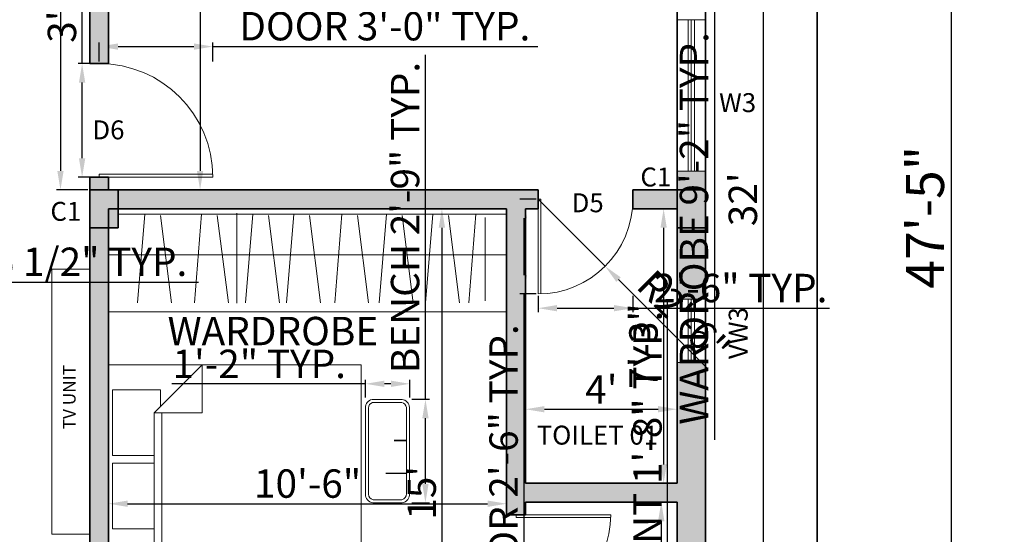
# Model space of a CAD drawing. Units: inches. Extents: x 4312 to 4955, y 6030 to 6717.
# Tile 3 of 5: x 4643 to 4955, y 6255 to 6418. Entities that reach past the tile are written whole.
import ezdxf

# ---------------------------------------------------------------- set-up
doc = ezdxf.new("R2010")
doc.units = ezdxf.units.IN
for name, color, linetype, lineweight in [('A-AREA-IDEN', 7, 'Continuous', 20), ('A-FLOR-CASE', 40, 'Continuous', 18), ('A-WALL', 7, 'Continuous', 35), ('C-PROP', 7, 'Continuous', 35), ('Dimensions', 112, 'Continuous', 13), ('Doors', 10, 'Continuous', 18), ('Furniture', 30, 'Continuous', 18), ('Text', 30, 'Continuous', 18), ('Windows', 160, 'Continuous', 18)]:
    doc.layers.add(name, color=color, linetype=linetype, lineweight=lineweight)
doc.layers.add('A-WALL-PATT', color=251, linetype='Continuous', lineweight=13, true_color=0x636466)
doc.layers.add('Column', color=52, linetype='Continuous', lineweight=35, true_color=0xc8c92d)
doc.styles.get("Standard").update_dxf_attribs({"font": 'arial.ttf'})
doc.dimstyles.new('ISO-25', dxfattribs={"dimtxt": 9, "dimasz": 6, "dimexe": 1.25, "dimexo": 0.625, "dimtad": 1, "dimdec": 1, "dimlunit": 3, "dimtxsty": 'Standard', "dimcen": 2.5, "dimadec": 0, "dimazin": 0, "dimtfac": 1, "dimtdec": 1, "dimtmove": 0, "dimatfit": 3, "dimfxl": 1, "dimarcsym": 0})

# ---------------------------------------------------------------- blocks, each defined once
blk = doc.blocks.new('D2')
at = {"layer": 'Doors'}
for p, q in [((4718.9, 6093.56), (4754.9, 6093.56)), ((4718.9, 6092.56), (4718.9, 6093.56)), ((4718.9, 6092.56), (4754.9, 6092.56))]:
    blk.add_line(p, q, dxfattribs=at)
blk.add_arc((4718.9, 6092.56), 36, 0, 90, dxfattribs=at)
blk = doc.blocks.new('D3')
at = {"layer": 'Doors'}
for p, q in [((5099.4, 6188.56), (5129.4, 6188.56)), ((5099.4, 6187.72), (5099.4, 6188.56)), ((5099.4, 6187.72), (5129.4, 6187.72))]:
    blk.add_line(p, q, dxfattribs=at)
blk.add_arc((5099.4, 6187.72), 30, 0, 90, dxfattribs=at)
blk = doc.blocks.new('W')
at = {"layer": 'Windows'}
for p, q in [((4457.75, 6177.72), (4457.75, 6168.72)), ((4505.75, 6177.72), (4505.75, 6168.72)), ((4457.75, 6174.22), (4505.75, 6174.22)), ((4457.75, 6173.22), (4505.75, 6173.22)), ((4457.75, 6172.22), (4505.75, 6172.22))]:
    blk.add_line(p, q, dxfattribs=at)
blk = doc.blocks.new('*D12')
at = {"layer": 'Defpoints', "color": 0, "transparency": 16777216}
for p in [(4655.8, 6543.72), (4655.8, 6363.72), (4665.05, 6363.72)]:
    blk.add_point(p, dxfattribs=at)
at = {"layer": 'Dimensions', "color": 0, "lineweight": -2, "transparency": 16777216}
for p, q in [((4656.43, 6543.72), (4657.05, 6543.72)), ((4655.8, 6537.72), (4655.8, 6369.72)), ((4664.42, 6363.72), (4654.55, 6363.72))]:
    blk.add_line(p, q, dxfattribs=at)
at = {"layer": 'Dimensions', "color": 0, "transparency": 16777216}
for points in [[(4654.8, 6537.72), (4656.8, 6537.72), (4655.8, 6543.72)], [(4654.8, 6369.72), (4656.8, 6369.72), (4655.8, 6363.72)]]:
    blk.add_solid(points, dxfattribs=at)
at = {"layer": 'Dimensions', "color": 0, "transparency": 16777216, "insert": (4650.58, 6453.72), "char_height": 9, "attachment_point": 5, "rotation": 90}
blk.add_mtext("15'", dxfattribs=at)
blk = doc.blocks.new('*D13')
at = {"layer": 'Defpoints', "color": 0, "transparency": 16777216}
for p in [(4690.28, 6543.72), (4690.28, 6363.72), (4700.01, 6363.72)]:
    blk.add_point(p, dxfattribs=at)
at = {"layer": 'Dimensions', "color": 0, "lineweight": -2, "transparency": 16777216}
for p, q in [((4690.91, 6543.72), (4701.26, 6543.72)), ((4700.01, 6537.72), (4700.01, 6369.72)), ((4690.91, 6363.72), (4701.26, 6363.72))]:
    blk.add_line(p, q, dxfattribs=at)
at = {"layer": 'Dimensions', "color": 0, "transparency": 16777216}
for points in [[(4699.01, 6537.72), (4701.01, 6537.72), (4700.01, 6543.72)], [(4699.01, 6369.72), (4701.01, 6369.72), (4700.01, 6363.72)]]:
    blk.add_solid(points, dxfattribs=at)
at = {"layer": 'Dimensions', "color": 0, "transparency": 16777216, "insert": (4694.79, 6453.72), "char_height": 9, "attachment_point": 5, "rotation": 90}
blk.add_mtext("15'", dxfattribs=at)
blk = doc.blocks.new('*D15')
at = {"layer": 'Defpoints', "color": 0, "transparency": 16777216}
for p in [(4844.05, 6357.72), (4844.05, 6270.72), (4846.78, 6270.72)]:
    blk.add_point(p, dxfattribs=at)
at = {"layer": 'Dimensions', "color": 0, "lineweight": -2, "transparency": 16777216}
for p, q in [((4844.67, 6357.72), (4848.03, 6357.72)), ((4846.78, 6351.72), (4846.78, 6276.72)), ((4844.67, 6270.72), (4848.03, 6270.72))]:
    blk.add_line(p, q, dxfattribs=at)
at = {"layer": 'Dimensions', "color": 0, "transparency": 16777216}
for points in [[(4845.78, 6351.72), (4847.78, 6351.72), (4846.78, 6357.72)], [(4845.78, 6276.72), (4847.78, 6276.72), (4846.78, 6270.72)]]:
    blk.add_solid(points, dxfattribs=at)
at = {"layer": 'Dimensions', "color": 0, "transparency": 16777216, "insert": (4841.56, 6314.22), "char_height": 9, "attachment_point": 5, "rotation": 90}
blk.add_mtext('7\'-3"', dxfattribs=at)
blk = doc.blocks.new('*D16')
at = {"layer": 'Defpoints', "color": 0, "transparency": 16777216}
for p in [(4851.05, 6294.2), (4803.05, 6285.78), (4851.05, 6285.78)]:
    blk.add_point(p, dxfattribs=at)
at = {"layer": 'Dimensions', "color": 0, "lineweight": -2, "transparency": 16777216}
for p, q in [((4803.05, 6286.41), (4803.05, 6295.45)), ((4851.05, 6286.41), (4851.05, 6295.45)), ((4809.05, 6294.2), (4845.05, 6294.2))]:
    blk.add_line(p, q, dxfattribs=at)
at = {"layer": 'Dimensions', "color": 0, "transparency": 16777216}
for points in [[(4809.05, 6295.2), (4809.05, 6293.2), (4803.05, 6294.2)], [(4845.05, 6295.2), (4845.05, 6293.2), (4851.05, 6294.2)]]:
    blk.add_solid(points, dxfattribs=at)
at = {"layer": 'Dimensions', "color": 0, "transparency": 16777216, "insert": (4827.05, 6299.32), "char_height": 9, "attachment_point": 5}
blk.add_mtext("4'", dxfattribs=at)
blk = doc.blocks.new('*D17')
at = {"layer": 'Defpoints', "color": 0, "transparency": 16777216}
for p in [(4846.78, 6264.72), (4846.03, 6177.72), (4846.78, 6177.72)]:
    blk.add_point(p, dxfattribs=at)
at = {"layer": 'Dimensions', "color": 0, "lineweight": -2, "transparency": 16777216}
for p, q in [((4846.16, 6264.72), (4844.78, 6264.72)), ((4846.03, 6258.72), (4846.03, 6183.72)), ((4846.16, 6177.72), (4844.78, 6177.72))]:
    blk.add_line(p, q, dxfattribs=at)
at = {"layer": 'Dimensions', "color": 0, "transparency": 16777216}
for points in [[(4845.03, 6258.72), (4847.03, 6258.72), (4846.03, 6264.72)], [(4845.03, 6183.72), (4847.03, 6183.72), (4846.03, 6177.72)]]:
    blk.add_solid(points, dxfattribs=at)
at = {"layer": 'Dimensions', "color": 0, "transparency": 16777216, "insert": (4840.81, 6221.22), "char_height": 9, "attachment_point": 5, "rotation": 90}
blk.add_mtext('7\'-3"', dxfattribs=at)
blk = doc.blocks.new('*D19')
at = {"layer": 'Defpoints', "color": 0, "transparency": 16777216}
for p in [(4774.62, 6357.72), (4774.62, 6177.72), (4776.57, 6177.72)]:
    blk.add_point(p, dxfattribs=at)
at = {"layer": 'Dimensions', "color": 0, "lineweight": -2, "transparency": 16777216}
for p, q in [((4775.24, 6357.72), (4777.82, 6357.72)), ((4776.57, 6351.72), (4776.57, 6183.72)), ((4775.24, 6177.72), (4777.82, 6177.72))]:
    blk.add_line(p, q, dxfattribs=at)
at = {"layer": 'Dimensions', "color": 0, "transparency": 16777216}
for points in [[(4775.57, 6351.72), (4777.57, 6351.72), (4776.57, 6357.72)], [(4775.57, 6183.72), (4777.57, 6183.72), (4776.57, 6177.72)]]:
    blk.add_solid(points, dxfattribs=at)
at = {"layer": 'Dimensions', "color": 0, "transparency": 16777216, "insert": (4771.35, 6267.72), "char_height": 9, "attachment_point": 5, "rotation": 90}
blk.add_mtext("15'", dxfattribs=at)
blk = doc.blocks.new('*D20')
at = {"layer": 'Defpoints', "color": 0, "transparency": 16777216}
for p in [(4671.05, 6270.12), (4797.05, 6270.12), (4797.05, 6264.26)]:
    blk.add_point(p, dxfattribs=at)
at = {"layer": 'Dimensions', "color": 0, "lineweight": -2, "transparency": 16777216}
for p, q in [((4671.05, 6269.5), (4671.05, 6263.01)), ((4797.05, 6269.5), (4797.05, 6263.01)), ((4677.05, 6264.26), (4791.05, 6264.26))]:
    blk.add_line(p, q, dxfattribs=at)
at = {"layer": 'Dimensions', "color": 0, "transparency": 16777216}
for points in [[(4677.05, 6265.26), (4677.05, 6263.26), (4671.05, 6264.26)], [(4791.05, 6265.26), (4791.05, 6263.26), (4797.05, 6264.26)]]:
    blk.add_solid(points, dxfattribs=at)
at = {"layer": 'Dimensions', "color": 0, "transparency": 16777216, "insert": (4734.05, 6269.48), "char_height": 9, "attachment_point": 5}
blk.add_mtext('10\'-6"', dxfattribs=at)
blk = doc.blocks.new('*D39')
at = {"layer": 'Defpoints', "color": 0, "transparency": 16777216}
for p in [(4857.98, 6552.72), (4864.3, 6168.72), (4878.26, 6168.72)]:
    blk.add_point(p, dxfattribs=at)
at = {"layer": 'Dimensions', "color": 0, "lineweight": -2, "transparency": 16777216}
for p, q in [((4858.6, 6552.72), (4879.51, 6552.72)), ((4878.26, 6546.72), (4878.26, 6174.72)), ((4864.93, 6168.72), (4879.51, 6168.72))]:
    blk.add_line(p, q, dxfattribs=at)
at = {"layer": 'Dimensions', "color": 0, "transparency": 16777216}
for points in [[(4877.26, 6546.72), (4879.26, 6546.72), (4878.26, 6552.72)], [(4877.26, 6174.72), (4879.26, 6174.72), (4878.26, 6168.72)]]:
    blk.add_solid(points, dxfattribs=at)
at = {"layer": 'Dimensions', "color": 0, "transparency": 16777216, "insert": (4873.03, 6360.72), "char_height": 9, "attachment_point": 5, "rotation": 90}
blk.add_mtext("32'", dxfattribs=at)
blk = doc.blocks.new('*D41')
at = {"layer": 'Defpoints', "color": 0, "transparency": 16777216}
for p in [(4895.36, 6639.55), (4895.36, 6070.55), (4937.83, 6070.55)]:
    blk.add_point(p, dxfattribs=at)
at = {"layer": 'Dimensions', "color": 0, "lineweight": -2, "transparency": 16777216}
for p, q in [((4895.99, 6639.55), (4939.08, 6639.55)), ((4937.83, 6633.55), (4937.83, 6076.55)), ((4895.99, 6070.55), (4939.08, 6070.55))]:
    blk.add_line(p, q, dxfattribs=at)
at = {"layer": 'Dimensions', "color": 0, "transparency": 16777216}
for points in [[(4936.83, 6633.55), (4938.83, 6633.55), (4937.83, 6639.55)], [(4936.83, 6076.55), (4938.83, 6076.55), (4937.83, 6070.55)]]:
    blk.add_solid(points, dxfattribs=at)
at = {"layer": 'Dimensions', "color": 0, "transparency": 16777216, "insert": (4931.11, 6355.05), "char_height": 12, "attachment_point": 5, "rotation": 90}
blk.add_mtext('47\'-5"', dxfattribs=at)
blk = doc.blocks.new('BED-QUEEN-PLAN')
for p, q in [((0, 0), (0, 80.00003)), ((7.99999, 78.80003), (28.79998, 78.80003)), ((7.99999, 65.60003), (7.99999, 78.80003)), ((28.79998, 78.80003), (28.79998, 65.60003)), ((31.19999, 78.80003), (51.99999, 78.80003)), ((31.19999, 65.60003), (31.19999, 78.80003)), ((51.99999, 78.80003), (51.99999, 63.60003)), ((59.99999, 80.00003), (59.99999, 0)), ((0, 65.60003), (44.8, 65.60003)), ((59.99999, 50.40003), (44.8, 65.60003)), ((44.8, 65.60003), (44.8, 50.40003)), ((44.8, 63.20003), (0, 63.20003)), ((51.99999, 63.60003), (46.79936, 63.60003)), ((44.8, 50.40003), (59.99999, 50.40003)), ((59.99999, 0), (0, 0))]:
    blk.add_line(p, q)
blk = doc.blocks.new('BEDROOM-BENCH')
for p, q in [((9.25, 1.01), (9.25, 7.57)), ((9.35, 1.01), (9.35, 7.57)), ((9.45, 1.01), (9.45, 7.57)), ((19.62, 1.01), (19.62, 4.91)), ((19.72, 1.01), (19.72, 4.91)), ((19.82, 1.01), (19.82, 4.91))]:
    blk.add_line(p, q)
blk.add_lwpolyline([(30.1, 13.99), (2.75, 13.99, 0.367048), (0, 11.66), (0, 2.33, 0.386896), (2.94, 0.01), (30.22, 0.01, 0.350808), (32.79, 2.35), (32.79, 11.9, 0.341474)], format="xyb", close=True)
blk.add_lwpolyline([(30.1, 12.99), (2.75, 12.99, 0.355496), (1, 11.56), (1, 2.42, 0.38014), (2.9, 1.01), (30.18, 1.01, 0.335385), (31.79, 2.44), (31.79, 11.76, 0.335385), (30.02, 12.99)], format="xyb")
blk = doc.blocks.new('VENT-WINDOW-20')
for p, q in [((0, 20), (9, 20)), ((3.5, 20), (3.5, 0)), ((4.5, 20), (4.5, 0)), ((5.5, 20), (5.5, 0)), ((9, 0), (0, 0))]:
    blk.add_line(p, q)
blk = doc.blocks.new('WARDROBE-HANGING-RAIL')
for p, q in [((0, 0.04), (2.27, 28.16)), ((17.98, 0.04), (20.26, 28.16)), ((31.43, 0), (31.43, 28.54)), ((34.18, 0.04), (36.45, 28.16)), ((47.17, 0.04), (49.44, 28.16)), ((62.41, 0.04), (64.68, 28.16)), ((76.5, 0.04), (78.77, 28.16)), ((91.21, 0.04), (93.48, 28.16)), ((104.86, 0.04), (107.13, 28.16)), ((7.23, 27.75), (10.74, 0.04)), ((25.22, 27.75), (28.73, 0.04)), ((41.41, 27.75), (44.92, 0.04)), ((54.4, 27.75), (57.91, 0.04)), ((69.64, 27.75), (73.15, 0.04)), ((83.73, 27.75), (87.24, 0.04)), ((98.44, 27.75), (101.95, 0.04)), ((110.06, 27.17), (110.06, 0.69))]:
    blk.add_line(p, q)
blk = doc.blocks.new('COLUMN-9X12-EDGE')
h = blk.add_hatch(color=256)
h.dxf.hatch_style = 1
h.paths.add_polyline_path([(9, 12), (0, 12), (0, 0), (9, 0)])
blk.add_lwpolyline([(9, 0), (0, 0)])
blk = doc.blocks.new('*D59')
at = {"layer": 'Defpoints', "color": 0, "transparency": 16777216}
for p in [(4704.05, 6409.12), (4668.05, 6403.72), (4704.05, 6403.72)]:
    blk.add_point(p, dxfattribs=at)
at = {"layer": 'Dimensions', "color": 0, "lineweight": -2, "transparency": 16777216}
for p, q in [((4668.05, 6404.35), (4668.05, 6410.37)), ((4704.05, 6404.35), (4704.05, 6410.37)), ((4674.05, 6409.12), (4698.05, 6409.12)), ((4704.05, 6409.12), (4806.92, 6409.12))]:
    blk.add_line(p, q, dxfattribs=at)
at = {"layer": 'Dimensions', "color": 0, "transparency": 16777216}
for points in [[(4674.05, 6410.12), (4674.05, 6408.12), (4668.05, 6409.12)], [(4698.05, 6410.12), (4698.05, 6408.12), (4704.05, 6409.12)]]:
    blk.add_solid(points, dxfattribs=at)
at = {"layer": 'Dimensions', "color": 0, "transparency": 16777216, "insert": (4758.49, 6414.41), "char_height": 9, "attachment_point": 5}
blk.add_mtext('DOOR 3\'-0" TYP.', dxfattribs=at)
blk = doc.blocks.new('*D60')
at = {"layer": 'Defpoints', "color": 0, "transparency": 16777216}
for p in [(4662.65, 6403.72), (4668.05, 6403.72), (4668.05, 6367.72)]:
    blk.add_point(p, dxfattribs=at)
at = {"layer": 'Dimensions', "color": 0, "lineweight": -2, "transparency": 16777216}
for p, q in [((4662.65, 6403.72), (4662.65, 6465.83)), ((4667.42, 6403.72), (4661.4, 6403.72)), ((4662.65, 6373.72), (4662.65, 6397.72)), ((4667.42, 6367.72), (4661.4, 6367.72))]:
    blk.add_line(p, q, dxfattribs=at)
at = {"layer": 'Dimensions', "color": 0, "transparency": 16777216}
for points in [[(4661.65, 6397.72), (4663.65, 6397.72), (4662.65, 6403.72)], [(4661.65, 6373.72), (4663.65, 6373.72), (4662.65, 6367.72)]]:
    blk.add_solid(points, dxfattribs=at)
at = {"layer": 'Dimensions', "color": 0, "transparency": 16777216, "insert": (4657.43, 6437.78), "char_height": 9, "attachment_point": 5, "rotation": 90}
blk.add_mtext('3\'-0" TYP.', dxfattribs=at)
blk = doc.blocks.new('*D61')
at = {"layer": 'Defpoints', "color": 0, "transparency": 16777216}
for p in [(4807.05, 6360.72), (4802.55, 6330.72), (4807.05, 6330.72)]:
    blk.add_point(p, dxfattribs=at)
at = {"layer": 'Dimensions', "color": 0, "lineweight": -2, "transparency": 16777216}
for p, q in [((4806.42, 6360.72), (4801.3, 6360.72)), ((4802.55, 6354.72), (4802.55, 6336.72)), ((4806.42, 6330.72), (4801.3, 6330.72)), ((4802.55, 6330.72), (4802.55, 6190.78))]:
    blk.add_line(p, q, dxfattribs=at)
at = {"layer": 'Dimensions', "color": 0, "transparency": 16777216}
for points in [[(4801.55, 6354.72), (4803.55, 6354.72), (4802.55, 6360.72)], [(4801.55, 6336.72), (4803.55, 6336.72), (4802.55, 6330.72)]]:
    blk.add_solid(points, dxfattribs=at)
at = {"layer": 'Dimensions', "color": 0, "transparency": 16777216, "insert": (4797.27, 6257.75), "char_height": 9, "attachment_point": 5, "rotation": 90}
blk.add_mtext('BATH DOOR 2\'-6" TYP.', dxfattribs=at)
blk = doc.blocks.new('*D62')
at = {"layer": 'Defpoints', "color": 0, "transparency": 16777216}
for p in [(4807.05, 6330.72), (4837.05, 6330.72), (4837.05, 6326.22)]:
    blk.add_point(p, dxfattribs=at)
at = {"layer": 'Dimensions', "color": 0, "lineweight": -2, "transparency": 16777216}
for p, q in [((4807.05, 6330.1), (4807.05, 6324.97)), ((4837.05, 6330.1), (4837.05, 6324.97)), ((4813.05, 6326.22), (4831.05, 6326.22)), ((4837.05, 6326.22), (4899.31, 6326.22))]:
    blk.add_line(p, q, dxfattribs=at)
at = {"layer": 'Dimensions', "color": 0, "transparency": 16777216}
for points in [[(4813.05, 6327.22), (4813.05, 6325.22), (4807.05, 6326.22)], [(4831.05, 6327.22), (4831.05, 6325.22), (4837.05, 6326.22)]]:
    blk.add_solid(points, dxfattribs=at)
at = {"layer": 'Dimensions', "color": 0, "transparency": 16777216, "insert": (4871.18, 6331.44), "char_height": 9, "attachment_point": 5}
blk.add_mtext('2\'-6" TYP.', dxfattribs=at)
blk = doc.blocks.new('*D65')
at = {"layer": 'Defpoints', "color": 0, "transparency": 16777216}
for p in [(4848.05, 6228.54), (4851.05, 6228.54), (4851.05, 6208.54)]:
    blk.add_point(p, dxfattribs=at)
at = {"layer": 'Dimensions', "color": 0, "lineweight": -2, "transparency": 16777216}
for p, q in [((4848.05, 6228.54), (4848.05, 6328.15)), ((4850.42, 6228.54), (4846.8, 6228.54)), ((4848.05, 6214.54), (4848.05, 6222.54)), ((4850.42, 6208.54), (4846.8, 6208.54))]:
    blk.add_line(p, q, dxfattribs=at)
at = {"layer": 'Dimensions', "color": 0, "transparency": 16777216}
for points in [[(4847.05, 6222.54), (4849.05, 6222.54), (4848.05, 6228.54)], [(4847.05, 6214.54), (4849.05, 6214.54), (4848.05, 6208.54)]]:
    blk.add_solid(points, dxfattribs=at)
at = {"layer": 'Dimensions', "color": 0, "transparency": 16777216, "insert": (4842.83, 6281.35), "char_height": 9, "attachment_point": 5, "rotation": 90}
blk.add_mtext('VENT 1\'-8" TYP.', dxfattribs=at)
blk = doc.blocks.new('*D75')
at = {"layer": 'Defpoints', "color": 0, "transparency": 16777216}
for p in [(4524.79, 6337.28), (4543.5, 6337.28), (4543.5, 6334.47)]:
    blk.add_point(p, dxfattribs=at)
at = {"layer": 'Dimensions', "color": 0, "lineweight": -2, "transparency": 16777216}
for p, q in [((4524.79, 6336.65), (4524.79, 6333.22)), ((4543.5, 6336.65), (4543.5, 6333.22)), ((4530.79, 6334.47), (4537.5, 6334.47)), ((4543.5, 6334.47), (4699.47, 6334.47))]:
    blk.add_line(p, q, dxfattribs=at)
at = {"layer": 'Dimensions', "color": 0, "transparency": 16777216}
for points in [[(4530.79, 6335.47), (4530.79, 6333.47), (4524.79, 6334.47)], [(4537.5, 6335.47), (4537.5, 6333.47), (4543.5, 6334.47)]]:
    blk.add_solid(points, dxfattribs=at)
at = {"layer": 'Dimensions', "color": 0, "transparency": 16777216, "insert": (4624.48, 6339.75), "char_height": 9, "attachment_point": 5}
blk.add_mtext('END TABLE 1\'-6 1/2" TYP.', dxfattribs=at)
blk = doc.blocks.new('*D77')
at = {"layer": 'Defpoints', "color": 0, "transparency": 16777216}
for p in [(4766.44, 6297.34), (4771.36, 6297.34), (4766.44, 6264.54)]:
    blk.add_point(p, dxfattribs=at)
at = {"layer": 'Dimensions', "color": 0, "lineweight": -2, "transparency": 16777216}
for p, q in [((4771.36, 6297.34), (4771.36, 6406.55)), ((4767.06, 6297.34), (4772.61, 6297.34)), ((4771.36, 6270.54), (4771.36, 6291.34)), ((4767.06, 6264.54), (4772.61, 6264.54))]:
    blk.add_line(p, q, dxfattribs=at)
at = {"layer": 'Dimensions', "color": 0, "transparency": 16777216}
for points in [[(4770.36, 6291.34), (4772.36, 6291.34), (4771.36, 6297.34)], [(4770.36, 6270.54), (4772.36, 6270.54), (4771.36, 6264.54)]]:
    blk.add_solid(points, dxfattribs=at)
at = {"layer": 'Dimensions', "color": 0, "transparency": 16777216, "insert": (4766.08, 6354.95), "char_height": 9, "attachment_point": 5, "rotation": 90}
blk.add_mtext('BENCH 2\'-9" TYP.', dxfattribs=at)
blk = doc.blocks.new('*D78')
at = {"layer": 'Defpoints', "color": 0, "transparency": 16777216}
for p in [(4752.36, 6302.26), (4752.36, 6297.34), (4766.44, 6297.34)]:
    blk.add_point(p, dxfattribs=at)
at = {"layer": 'Dimensions', "color": 0, "lineweight": -2, "transparency": 16777216}
for p, q in [((4752.36, 6302.26), (4691.09, 6302.26)), ((4752.36, 6297.96), (4752.36, 6303.51)), ((4760.44, 6302.26), (4758.36, 6302.26)), ((4766.44, 6297.96), (4766.44, 6303.51))]:
    blk.add_line(p, q, dxfattribs=at)
at = {"layer": 'Dimensions', "color": 0, "transparency": 16777216}
for points in [[(4758.36, 6303.26), (4758.36, 6301.26), (4752.36, 6302.26)], [(4760.44, 6303.26), (4760.44, 6301.26), (4766.44, 6302.26)]]:
    blk.add_solid(points, dxfattribs=at)
at = {"layer": 'Dimensions', "color": 0, "transparency": 16777216, "insert": (4718.73, 6307.4), "char_height": 9, "attachment_point": 5}
blk.add_mtext('1\'-2" TYP.', dxfattribs=at)
blk = doc.blocks.new('*D79')
at = {"layer": 'Defpoints', "color": 0, "transparency": 16777216}
for p in [(4846.33, 6534.56), (4846.33, 6424.5), (4862.84, 6424.5)]:
    blk.add_point(p, dxfattribs=at)
at = {"layer": 'Dimensions', "color": 0, "lineweight": -2, "transparency": 16777216}
for p, q in [((4846.95, 6534.56), (4864.09, 6534.56)), ((4862.84, 6528.56), (4862.84, 6430.5)), ((4846.95, 6424.5), (4864.09, 6424.5)), ((4862.84, 6424.5), (4862.84, 6284.48))]:
    blk.add_line(p, q, dxfattribs=at)
at = {"layer": 'Dimensions', "color": 0, "transparency": 16777216}
for points in [[(4861.84, 6528.56), (4863.84, 6528.56), (4862.84, 6534.56)], [(4861.84, 6430.5), (4863.84, 6430.5), (4862.84, 6424.5)]]:
    blk.add_solid(points, dxfattribs=at)
at = {"layer": 'Dimensions', "color": 0, "transparency": 16777216, "insert": (4857.56, 6351.49), "char_height": 9, "attachment_point": 5, "rotation": 90}
blk.add_mtext('WARDROBE 9\'-2" TYP.', dxfattribs=at)
blk = doc.blocks.new('*D88')
at = {"layer": 'Defpoints', "color": 0, "transparency": 16777216}
for p in [(4895.36, 6639.55), (4860.05, 6552.72), (4895.36, 6038.3)]:
    blk.add_point(p, dxfattribs=at)
at = {"layer": 'Dimensions', "color": 0, "lineweight": -2, "transparency": 16777216}
for p, q in [((4895.36, 6638.92), (4895.36, 6037.05)), ((4860.05, 6552.1), (4860.05, 6037.05)), ((4866.05, 6038.3), (4889.36, 6038.3)), ((4895.36, 6038.3), (4954.65, 6038.3))]:
    blk.add_line(p, q, dxfattribs=at)
at = {"layer": 'Dimensions', "color": 0, "transparency": 16777216}
for points in [[(4866.05, 6039.3), (4866.05, 6037.3), (4860.05, 6038.3)], [(4889.36, 6039.3), (4889.36, 6037.3), (4895.36, 6038.3)]]:
    blk.add_solid(points, dxfattribs=at)
at = {"layer": 'Dimensions', "color": 0, "transparency": 16777216, "insert": (4928.01, 6043.58), "char_height": 9, "attachment_point": 5}
blk.add_mtext('2\'-11 1/2"', dxfattribs=at)
blk = doc.blocks.new('*D96')
at = {"layer": 'Defpoints', "color": 0, "transparency": 16777216}
for p in [(4807.05, 6360.72), (4828.26, 6339.51)]:
    blk.add_point(p, dxfattribs=at)
at = {"layer": 'Dimensions', "color": 0, "lineweight": -2, "transparency": 16777216}
for p, q in [((4807.05, 6360.72), (4828.26, 6339.51)), ((4860.64, 6307.13), (4832.5, 6335.27))]:
    blk.add_line(p, q, dxfattribs=at)
at = {"layer": 'Dimensions', "color": 0, "transparency": 16777216}
blk.add_solid([(4833.21, 6335.98), (4831.8, 6334.56), (4828.26, 6339.51)], dxfattribs=at)
at = {"layer": 'Dimensions', "color": 0, "transparency": 16777216, "insert": (4852.38, 6322.77), "char_height": 9, "attachment_point": 5, "rotation": 314.9991}
blk.add_mtext('R2\'-6"', dxfattribs=at)

msp = doc.modelspace()

# ---------------------------------------------------------------- hatches: boundary and pattern name
at = {"layer": 'A-WALL-PATT'}
h = msp.add_hatch(color=256, dxfattribs=at)
h.dxf.hatch_style = 1
h.paths.add_polyline_path([(4671.05, 6543.72), (4665.05, 6543.72), (4665.05, 6403.72), (4671.05, 6403.72)])
h = msp.add_hatch(color=256, dxfattribs=at)
h.dxf.hatch_style = 1
h.paths.add_polyline_path([(4860.05, 6369.64), (4851.05, 6369.64), (4851.05, 6363.72), (4860.05, 6363.72)])
h = msp.add_hatch(color=256, dxfattribs=at)
h.dxf.hatch_style = 1
h.paths.add_polyline_path([(4671.05, 6367.72), (4665.05, 6367.72), (4665.05, 6363.72), (4671.05, 6363.72)])
h = msp.add_hatch(color=256, dxfattribs=at)
h.dxf.hatch_style = 1
h.paths.add_polyline_path([(4860.05, 6309.06), (4851.05, 6309.06), (4851.05, 6270.72), (4803.05, 6270.72), (4803.05, 6357.72), (4807.05, 6357.72), (4807.05, 6363.72), (4674.05, 6363.72), (4674.05, 6357.72), (4797.05, 6357.72), (4797.05, 6260.72), (4803.05, 6260.72), (4803.05, 6264.72), (4851.05, 6264.72), (4851.05, 6228.54), (4860.05, 6228.54)])
h = msp.add_hatch(color=256, dxfattribs=at)
h.dxf.hatch_style = 1
h.paths.add_polyline_path([(4851.05, 6363.72), (4837.05, 6363.72), (4837.05, 6357.72), (4851.05, 6357.72)], flags=17)
h = msp.add_hatch(color=256, dxfattribs=at)
h.dxf.hatch_style = 1
h.paths.add_polyline_path([(4671.05, 6351.72), (4665.05, 6351.72), (4665.05, 6223.72), (4671.05, 6223.72)])
h = msp.add_hatch(color=256, dxfattribs=at)
h.dxf.hatch_style = 1
h.paths.add_polyline_path([(4860.05, 6351.72), (4851.05, 6351.72), (4851.05, 6329.06), (4860.05, 6329.06)], flags=17)
at = {"layer": 'Column'}
h = msp.add_hatch(color=256, dxfattribs=at)
h.dxf.hatch_style = 1
h.paths.add_polyline_path([(4671.05, 6351.72), (4674.05, 6351.72), (4674.05, 6357.72), (4674.05, 6363.72), (4665.05, 6363.72), (4665.05, 6351.72)])

# ---------------------------------------------------------------- linework, layer by layer
at = {"layer": 'A-FLOR-CASE'}
for p, q in [((4674.05, 6355.99), (4797.05, 6355.99)), ((4797.05, 6343.09), (4671.05, 6343.09)), ((4665.05, 6338.6), (4653.05, 6338.6)), ((4653.05, 6338.6), (4653.05, 6254.6)), ((4671.05, 6325.09), (4797.05, 6325.09)), ((4653.05, 6254.6), (4665.05, 6254.6))]:
    msp.add_line(p, q, dxfattribs=at)
at = {"layer": 'A-WALL'}
for p, q in [((4860.05, 6552.72), (4860.05, 6090.72)), ((4665.05, 6543.72), (4665.05, 6403.72)), ((4671.05, 6543.72), (4671.05, 6403.72)), ((4851.05, 6543.72), (4851.05, 6270.72)), ((4665.05, 6403.72), (4671.05, 6403.72)), ((4665.05, 6367.72), (4671.05, 6367.72)), ((4665.05, 6367.72), (4665.05, 6223.72)), ((4671.05, 6367.72), (4671.05, 6363.72)), ((4671.05, 6363.72), (4807.05, 6363.72)), ((4807.05, 6363.72), (4807.05, 6357.72)), ((4837.05, 6363.72), (4837.05, 6357.72)), ((4837.05, 6363.72), (4860.05, 6363.72)), ((4671.05, 6357.72), (4797.05, 6357.72)), ((4671.05, 6357.72), (4671.05, 6223.72)), ((4797.05, 6357.72), (4797.05, 6260.72)), ((4803.05, 6357.72), (4803.05, 6270.72)), ((4803.05, 6357.72), (4807.05, 6357.72)), ((4837.05, 6357.72), (4851.05, 6357.72)), ((4803.05, 6270.72), (4851.05, 6270.72)), ((4803.05, 6264.72), (4851.05, 6264.72)), ((4803.05, 6264.72), (4803.05, 6260.72)), ((4851.05, 6264.72), (4851.05, 6177.72)), ((4797.05, 6260.72), (4803.05, 6260.72))]:
    msp.add_line(p, q, dxfattribs=at)
at = {"layer": 'C-PROP'}
msp.add_lwpolyline([(4895.36, 6639.55), (4895.36, 6070.55), (4355.36, 6070.55), (4379.36, 6639.55)], close=True, dxfattribs=at)
at = {"layer": 'Column'}
msp.add_lwpolyline([(4665.05, 6363.72), (4674.05, 6363.72), (4674.05, 6351.72), (4665.05, 6351.72)], close=True, dxfattribs=at)

# ---------------------------------------------------------------- block references
at = {"layer": 'A-FLOR-CASE'}
msp.add_blockref('WARDROBE-HANGING-RAIL', (4680.22, 6327.83), dxfattribs=at)
at = {"layer": 'Column'}
msp.add_blockref('COLUMN-9X12-EDGE', (4851.05, 6351.72), dxfattribs=at)
at = {"layer": 'Doors'}
msp.add_blockref('D2', (-50.85, 275.16), dxfattribs=at)
at = {"layer": 'Doors', "rotation": 270}
msp.add_blockref('D3', (-1380.68, 11460.13), dxfattribs=at)
at = {"layer": 'Doors', "xscale": -1, "rotation": 180}
msp.add_blockref('D3', (-299.35, 12448.45), dxfattribs=at)
at = {"layer": 'Furniture'}
for name, p, rotation in [('BED-QUEEN-PLAN', (4751.05, 6248.3), 90.00000000000134), ('BEDROOM-BENCH', (4766.34, 6264.54), 89.99999999993678)]:
    msp.add_blockref(name, p, dxfattribs=dict(at, rotation=rotation))
at = {"layer": 'Windows', "rotation": 270}
msp.add_blockref('W', (-1317.68, 10875.39), dxfattribs=at)
at = {"layer": 'Windows'}
msp.add_blockref('VENT-WINDOW-20', (4851.05, 6309.06), dxfattribs=at)

# ---------------------------------------------------------------- texts
at = {"layer": 'A-AREA-IDEN', "insert": (4806.59, 6288.99), "char_height": 6, "attachment_point": 1, "rotation": 0.0025}
msp.add_mtext_dynamic_manual_height_columns('TOILET 01', width=65.4832, gutter_width=12.5, heights=[0], dxfattribs=at)
at = {"layer": 'Text', "char_height": 6, "attachment_point": 1}
for s, insert in [('W3', (4864.34, 6394.35)), ('D6', (4665.89, 6385.72)), ('C1', (4839.43, 6370.79)), ('D5', (4817.64, 6362.62)), ('C1', (4652.62, 6359.9))]:
    msp.add_mtext_dynamic_manual_height_columns(s, width=4.4911, gutter_width=12.5, heights=[0], dxfattribs=dict(at, insert=insert))
at = {"layer": 'Text', "attachment_point": 1}
for s, width, insert, char_height, rotation in [('VW3', 19.9533, (4867.39, 6310.09), 6, 90), ('WARDROBE', 89.0701, (4689.71, 6323.47), 9, 0.0025), ('TV UNIT', 25.2838, (4656.57, 6287.85), 4, 90)]:
    msp.add_mtext_dynamic_manual_height_columns(s, width=width, gutter_width=12.5, heights=[0], dxfattribs=dict(at, insert=insert, char_height=char_height, rotation=rotation))

# ---------------------------------------------------------------- dimensions: what is measured, and where the dimension line sits
at = {"layer": 'Dimensions'}
for base, p1, p2, override, picture, middle in [((4895.36, 6038.3), (4860.05, 6552.72), (4895.36, 6639.55), {"dimdec": 1, "dimlfac": 1, "dimrnd": 0, "dimzin": 1, "dimdsep": 46, "dimlunit": 4, "dimfrac": 2}, '*D88', (4928.01, 6043.58)), ((4851.05, 6294.2), (4803.05, 6285.78), (4851.05, 6285.78), {"dimclrd": 0, "dimclre": 0, "dimclrt": 0}, '*D16', (4827.05, 6299.32)), ((4797.05, 6264.26), (4671.05, 6270.12), (4797.05, 6270.12), {"dimclrd": 0, "dimclre": 0, "dimclrt": 0}, '*D20', (4734.05, 6269.48))]:
    dim = msp.add_linear_dim(base=base, p1=p1, p2=p2, dimstyle='ISO-25', override=override, dxfattribs=at)
    dim.commit()
    dim.dimension.update_dxf_attribs({"geometry": picture, "text_midpoint": middle})
for base, p1, p2, override, picture, middle in [((4937.83, 6070.55), (4895.36, 6639.55), (4895.36, 6070.55), {"dimtxt": 12, "dimclrd": 0, "dimclre": 0, "dimclrt": 0}, '*D41', (4931.11, 6355.05)), ((4878.26, 6168.72), (4857.98, 6552.72), (4864.3, 6168.72), {"dimclrd": 0, "dimclre": 0, "dimclrt": 0}, '*D39', (4873.03, 6360.72)), ((4655.8, 6363.72), (4655.8, 6543.72), (4665.05, 6363.72), {"dimclrd": 0, "dimclre": 0, "dimclrt": 0}, '*D12', (4650.58, 6453.72)), ((4700.01, 6363.72), (4690.28, 6543.72), (4690.28, 6363.72), {"dimclrd": 0, "dimclre": 0, "dimclrt": 0}, '*D13', (4694.79, 6453.72)), ((4776.57, 6177.72), (4774.62, 6357.72), (4774.62, 6177.72), {"dimclrd": 0, "dimclre": 0, "dimclrt": 0}, '*D19', (4771.35, 6267.72)), ((4846.78, 6270.72), (4844.05, 6357.72), (4844.05, 6270.72), {"dimclrd": 0, "dimclre": 0, "dimclrt": 0}, '*D15', (4841.56, 6314.22)), ((4846.03, 6177.72), (4846.78, 6264.72), (4846.78, 6177.72), {"dimclrd": 0, "dimclre": 0, "dimclrt": 0}, '*D17', (4840.81, 6221.22))]:
    dim = msp.add_linear_dim(base=base, p1=p1, p2=p2, angle=90, dimstyle='ISO-25', override=override, dxfattribs=at)
    dim.commit()
    dim.dimension.update_dxf_attribs({"geometry": picture, "text_midpoint": middle})
for base, p1, p2, angle, text, picture, middle in [((4862.84, 6424.5), (4846.33, 6534.56), (4846.33, 6424.5), 270, 'WARDROBE <> TYP.', '*D79', (4857.56, 6351.49)), ((4662.65, 6403.72), (4668.05, 6367.72), (4668.05, 6403.72), 90, '<> TYP.', '*D60', (4657.43, 6437.78)), ((4771.36, 6297.34), (4766.44, 6264.54), (4766.44, 6297.34), 90, 'BENCH <> TYP.', '*D77', (4766.08, 6354.95)), ((4802.55, 6330.72), (4807.05, 6360.72), (4807.05, 6330.72), 270, 'BATH DOOR <> TYP.', '*D61', (4797.27, 6257.75)), ((4848.05, 6228.54), (4851.05, 6208.54), (4851.05, 6228.54), 90, 'VENT <> TYP.', '*D65', (4842.83, 6281.35)), ((4752.36, 6302.26), (4766.44, 6297.34), (4752.36, 6297.34), 180, '<> TYP.', '*D78', (4718.73, 6307.4))]:
    dim = msp.add_linear_dim(base=base, p1=p1, p2=p2, angle=angle, text=text, dimstyle='ISO-25', override={"dimdec": 1, "dimlfac": 1, "dimrnd": 0, "dimzin": 1, "dimdsep": 46, "dimlunit": 4, "dimfrac": 2}, dxfattribs=at)
    dim.commit()
    dim.dimension.update_dxf_attribs({"geometry": picture, "text_midpoint": middle})
for base, p1, p2, text, picture, middle in [((4704.05, 6409.12), (4668.05, 6403.72), (4704.05, 6403.72), 'DOOR <> TYP.', '*D59', (4758.49, 6414.41)), ((4543.5, 6334.47), (4524.79, 6337.28), (4543.5, 6337.28), 'END TABLE <> TYP.', '*D75', (4624.48, 6339.75)), ((4837.05, 6326.22), (4807.05, 6330.72), (4837.05, 6330.72), '<> TYP.', '*D62', (4871.18, 6331.44))]:
    dim = msp.add_linear_dim(base=base, p1=p1, p2=p2, text=text, dimstyle='ISO-25', override={"dimdec": 1, "dimlfac": 1, "dimrnd": 0, "dimzin": 1, "dimdsep": 46, "dimlunit": 4, "dimfrac": 2}, dxfattribs=at)
    dim.commit()
    dim.dimension.update_dxf_attribs({"geometry": picture, "text_midpoint": middle})
dim = msp.add_radius_dim(center=(4807.05, 6360.72), mpoint=(4828.26, 6339.51), dimstyle='ISO-25', override={"dimdec": 1, "dimlfac": 1, "dimrnd": 0, "dimzin": 1, "dimdsep": 46, "dimlunit": 4, "dimfrac": 2}, dxfattribs=at)
dim.commit()
dim.dimension.update_dxf_attribs({"geometry": '*D96', "text_midpoint": (4852.38, 6322.77)})

doc.saveas('drawing.dxf')
